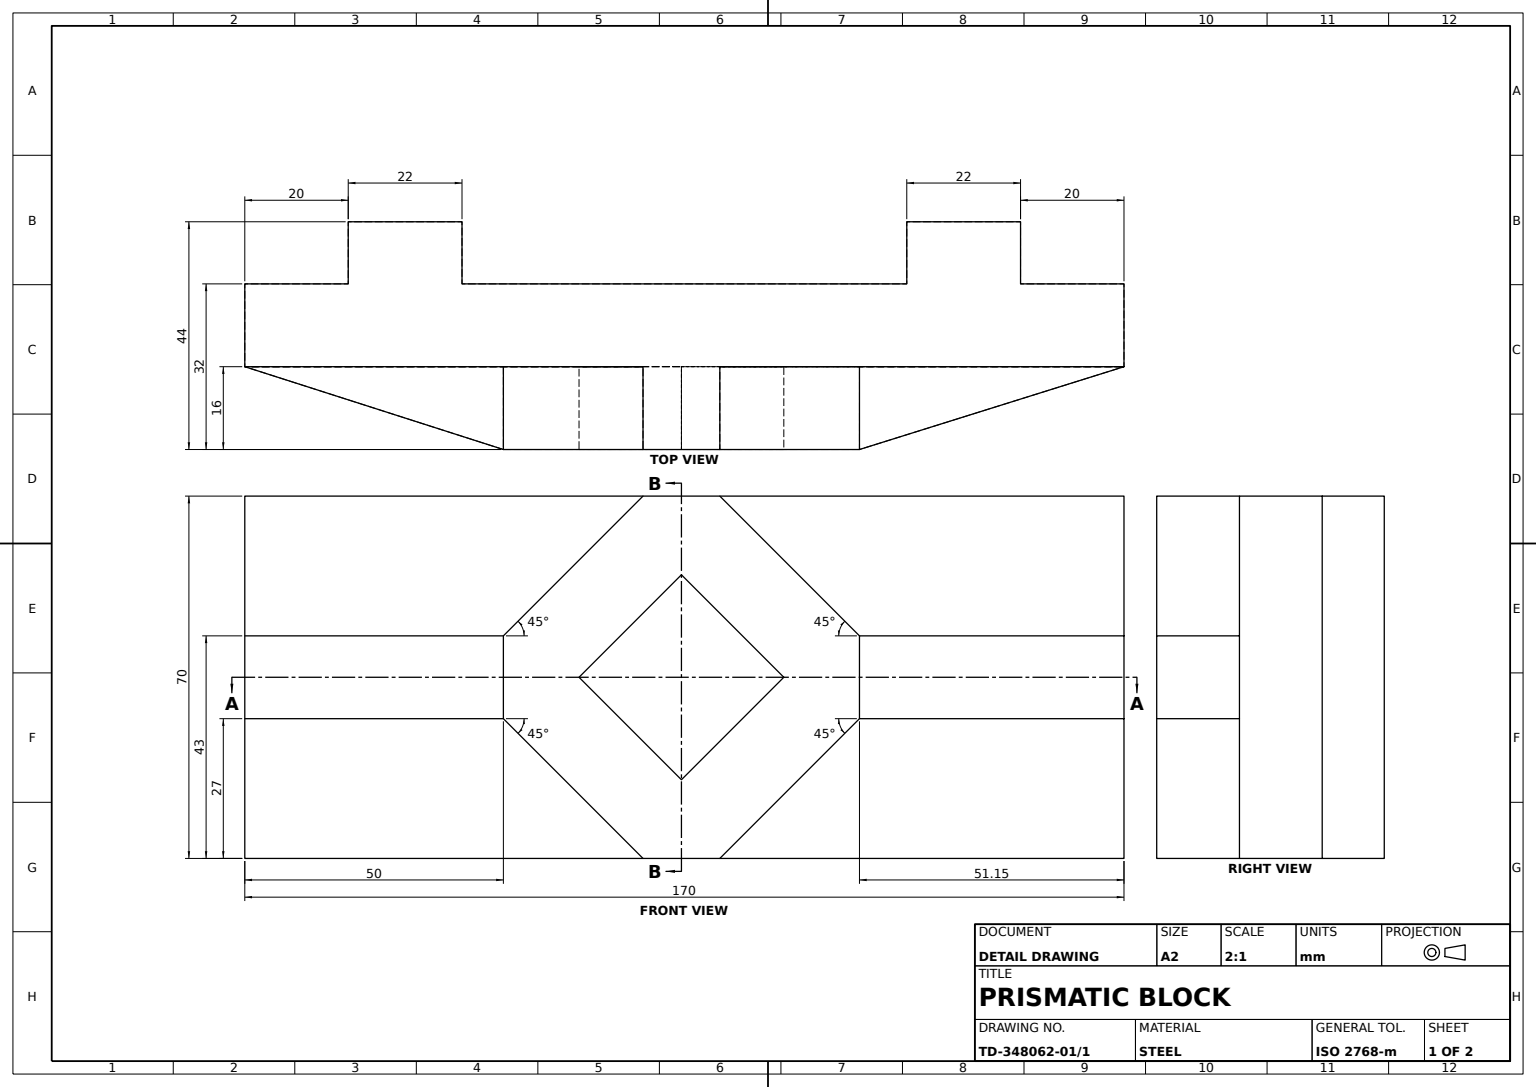
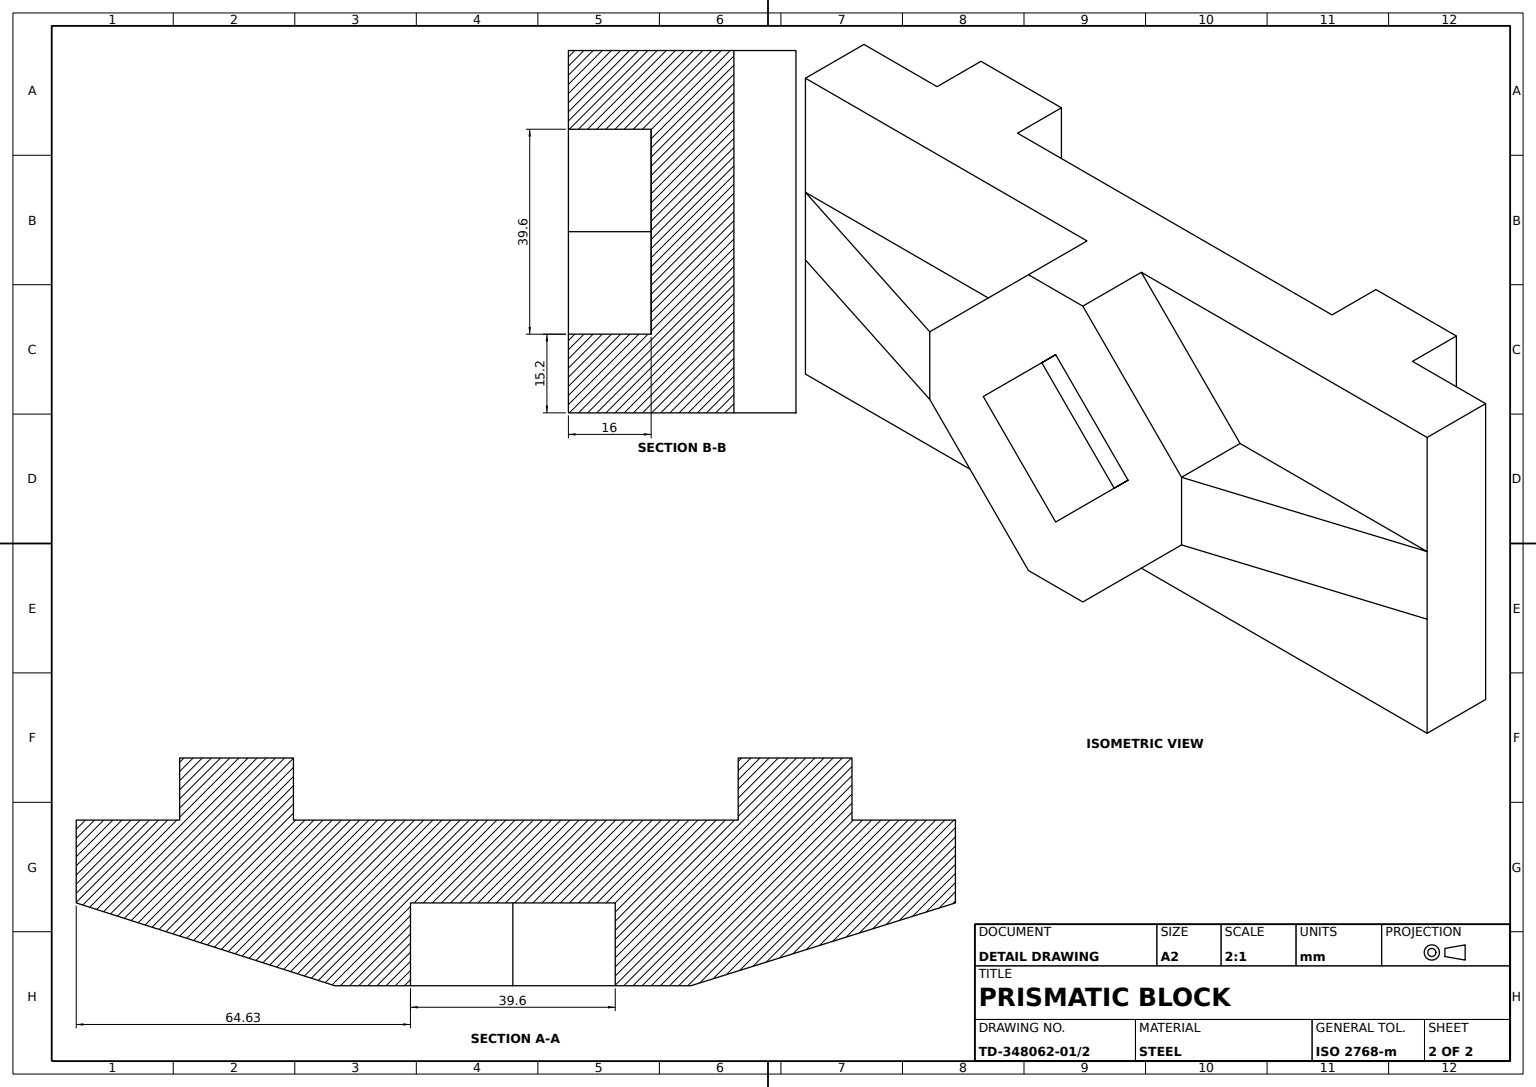
from build123d import *

# Parameters (mm, degrees)
BASE_PLATE_SKETCH_W      = 170
BASE_PLATE_SKETCH_H      = 70
BASE_PLATE_16MM_DEPTH    = 16
CENTER_BOSS_60X60_DEPTH  = 16
CENTER_POCKET_28_DEPTH   = 16
LEFT_WEDGE_BOSS_DEPTH    = 43
LEFT_WEDGE_CUT_DEPTH     = 27
RIGHT_WEDGE_BOSS_DEPTH   = 43
RIGHT_WEDGE_CUT_DEPTH    = 27
TOP_RAIL_SKETCH_W        = 22
TOP_RAIL_SKETCH_H        = 12
TOP_RAIL_WITH_TABS_DEPTH = 70


with BuildPart() as part:
    # Base Plate Sketch → Base Plate 16mm (new body)
    with BuildSketch(Plane.XY):
        with Locations((85, 35)):
            Rectangle(BASE_PLATE_SKETCH_W, BASE_PLATE_SKETCH_H)
    extrude(amount=BASE_PLATE_16MM_DEPTH)

    # Center Boss Sketch → Center Boss 60x60 (add)
    with BuildSketch(Plane.XY.offset(16)):
        Polygon((91.852813742, 70), (85, 70), (77, 70), (50, 43), (50, 35), (50, 27), (77, 0), (85, 0), (91.852813742, 0), (118.852813742, 27), (118.852813742, 35), (118.852813742, 43), align=None)
    extrude(amount=CENTER_BOSS_60X60_DEPTH)

    # Center Pocket Sketch → Center Pocket 28 (cut)
    with BuildSketch(Plane.XY.offset(32)):
        Polygon((84.426406871, 15.201010127), (104.225396744, 35), (84.426406871, 54.798989873), (64.627416998, 35), align=None)
    extrude(amount=-CENTER_POCKET_28_DEPTH, mode=Mode.SUBTRACT)

    # Left Wedge Sketch → Left Wedge Boss (add)
    with BuildSketch(Plane.XZ):
        Polygon((118.852813742, 32), (118.852813742, 16), (170, 16), align=None)
    extrude(amount=-LEFT_WEDGE_BOSS_DEPTH)

    # Left Wedge Cut Sketch → Left Wedge Cut (cut)
    with BuildSketch(Plane.XZ):
        Polygon((118.852813742, 32), (118.852813742, 16), (170, 16), align=None)
    extrude(amount=-LEFT_WEDGE_CUT_DEPTH, mode=Mode.SUBTRACT)

    # Right Wedge Sketch → Right Wedge Boss (add)
    with BuildSketch(Plane.XZ):
        Polygon((50, 32), (50, 16), (0, 16), align=None)
    extrude(amount=-RIGHT_WEDGE_BOSS_DEPTH)

    # Right Wedge Cut Sketch → Right Wedge Cut (cut)
    with BuildSketch(Plane.XZ):
        Polygon((50, 32), (50, 16), (0, 16), align=None)
    extrude(amount=-RIGHT_WEDGE_CUT_DEPTH, mode=Mode.SUBTRACT)

    # Top Rail Sketch → Top Rail with Tabs (add)
    with BuildSketch(Plane.XZ):
        with Locations((31, -6)):
            Rectangle(TOP_RAIL_SKETCH_W, TOP_RAIL_SKETCH_H)
        with Locations((139, -6)):
            Rectangle(TOP_RAIL_SKETCH_W, TOP_RAIL_SKETCH_H)
    extrude(amount=-TOP_RAIL_WITH_TABS_DEPTH)


solid = part.part
